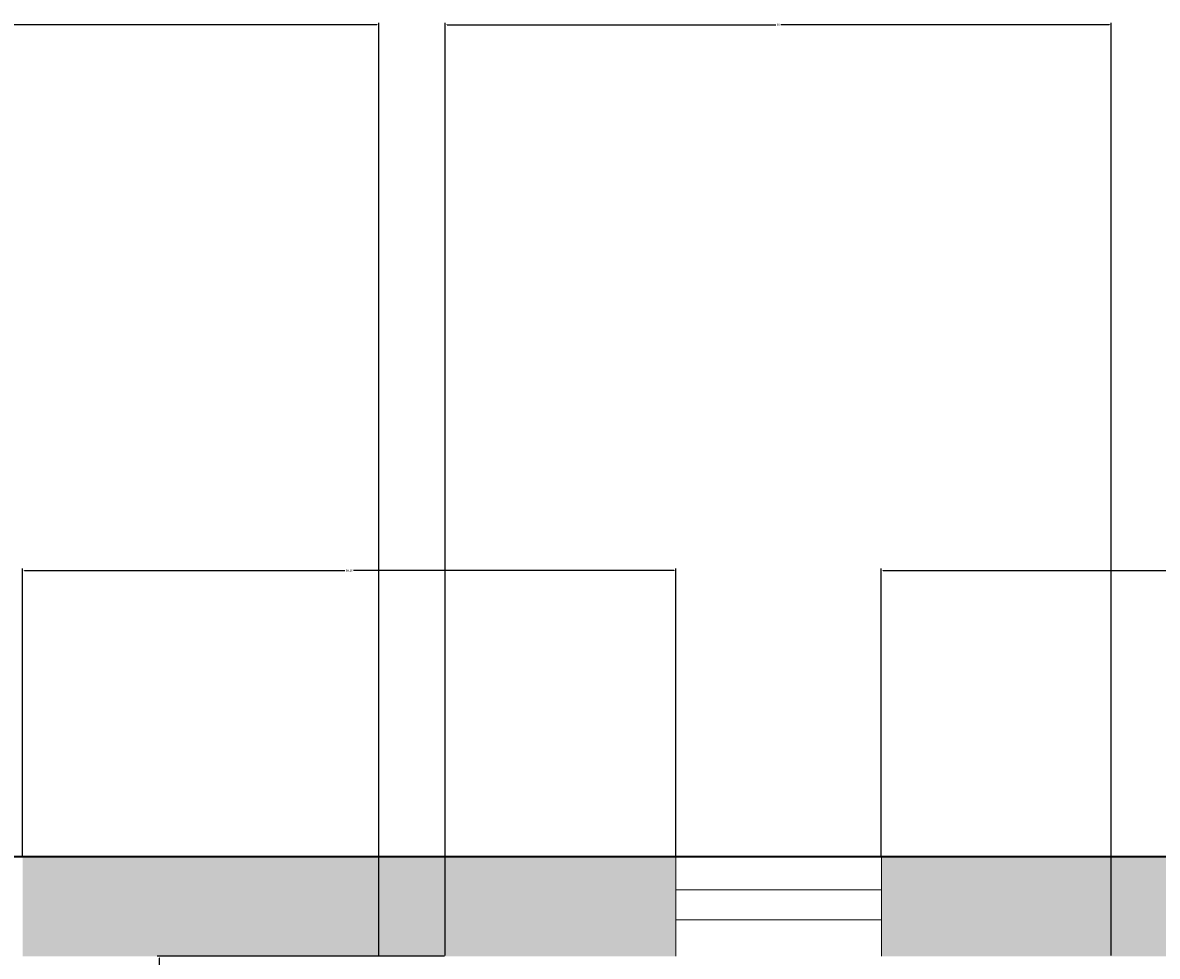
# Model space of a CAD drawing. Units: inches. Extents: x 3024 to 3952, y 1308 to 1863.
# Tile 24 of 29: x 3195 to 3297, y 1779 to 1863. Entities that reach past the tile are written whole.
import ezdxf

# ---------------------------------------------------------------- set-up
doc = ezdxf.new("R2010")
doc.units = ezdxf.units.IN
for name, color, linetype, lineweight in [('A-ANNO-DIMS', 2, 'Continuous', 18), ('A-GLAZ', 4, 'Continuous', 18), ('A-WALL', 7, 'Continuous', 35)]:
    doc.layers.add(name, color=color, linetype=linetype, lineweight=lineweight)
doc.layers.add('A-WALL-PATT', color=254, linetype='Continuous', lineweight=13, true_color=0xcecce6)
doc.styles.get("Standard").update_dxf_attribs({"font": 'arial.ttf'})
doc.dimstyles.get("Standard").update_dxf_attribs({"dimtxt": 0.18, "dimasz": 0.18, "dimexe": 0.18, "dimexo": 0.0625, "dimgap": 0.09, "dimtad": 0, "dimtih": 1, "dimtoh": 1, "dimdec": 4, "dimzin": 0, "dimdsep": 46, "dimtxsty": 'Standard', "dimcen": 0.09, "dimadec": 0, "dimazin": 0, "dimtfac": 1, "dimtdec": 4, "dimtofl": 0, "dimtmove": 0, "dimatfit": 3, "dimfxl": 1, "dimtolj": 1, "dimtzin": 0, "dimarcsym": 0})

# ---------------------------------------------------------------- blocks, each defined once
blk = doc.blocks.new('WIN-BATH-18p5IN')
for p, q in [((0, 5.99), (0, 9)), ((18.52, 6.41), (18.52, 9)), ((18.52, 6.41), (18.52, 5.99)), ((0, 3.28), (0, 0)), ((18.52, 3.69), (18.52, 0))]:
    blk.add_line(p, q)
blk.add_lwpolyline([(0, 5.99), (18.52, 5.99), (18.52, 3.28), (0, 3.28)], close=True)
blk = doc.blocks.new('*D38')
at = {"layer": 'A-ANNO-DIMS', "color": 0, "lineweight": -2, "transparency": 16777216}
for p, q in [((3106.76, 1778.67), (3106.76, 1862.78)), ((3226.76, 1778.67), (3226.76, 1862.78)), ((3106.94, 1862.6), (3166.48, 1862.6)), ((3226.58, 1862.6), (3167.04, 1862.6))]:
    blk.add_line(p, q, dxfattribs=at)
at = {"layer": 'A-ANNO-DIMS', "color": 0, "transparency": 16777216}
for points in [[(3106.94, 1862.63), (3106.94, 1862.57), (3106.76, 1862.6)], [(3226.58, 1862.63), (3226.58, 1862.57), (3226.76, 1862.6)]]:
    blk.add_solid(points, dxfattribs=at)
at = {"layer": 'Defpoints', "color": 0, "transparency": 16777216}
for p in [(3226.76, 1862.6), (3106.76, 1778.61), (3226.76, 1778.61)]:
    blk.add_point(p, dxfattribs=at)
at = {"layer": 'A-ANNO-DIMS', "color": 0, "transparency": 16777216, "insert": (3166.76, 1862.6), "char_height": 0.18, "attachment_point": 5}
blk.add_mtext('\\A1;120', dxfattribs=at)
blk = doc.blocks.new('*D39')
at = {"layer": 'A-ANNO-DIMS', "color": 0, "lineweight": -2, "transparency": 16777216}
for p, q in [((3232.76, 1778.67), (3232.76, 1862.78)), ((3292.76, 1778.67), (3292.76, 1862.78)), ((3232.94, 1862.6), (3262.54, 1862.6)), ((3292.58, 1862.6), (3262.98, 1862.6))]:
    blk.add_line(p, q, dxfattribs=at)
at = {"layer": 'A-ANNO-DIMS', "color": 0, "transparency": 16777216}
for points in [[(3232.94, 1862.63), (3232.94, 1862.57), (3232.76, 1862.6)], [(3292.58, 1862.63), (3292.58, 1862.57), (3292.76, 1862.6)]]:
    blk.add_solid(points, dxfattribs=at)
at = {"layer": 'Defpoints', "color": 0, "transparency": 16777216}
for p in [(3292.76, 1862.6), (3232.76, 1778.61), (3292.76, 1778.61)]:
    blk.add_point(p, dxfattribs=at)
at = {"layer": 'A-ANNO-DIMS', "color": 0, "transparency": 16777216, "insert": (3262.76, 1862.6), "char_height": 0.18, "attachment_point": 5}
blk.add_mtext('\\A1;60', dxfattribs=at)
blk = doc.blocks.new('*D51')
at = {"layer": 'A-ANNO-DIMS', "color": 0, "lineweight": -2, "transparency": 16777216}
for p, q in [((3232.7, 1778.61), (3206.81, 1778.61)), ((3206.99, 1778.43), (3206.99, 1736.79)), ((3206.99, 1694.79), (3206.99, 1736.42)), ((3232.7, 1694.61), (3206.81, 1694.61))]:
    blk.add_line(p, q, dxfattribs=at)
at = {"layer": 'A-ANNO-DIMS', "color": 0, "transparency": 16777216}
for points in [[(3206.96, 1778.43), (3207.02, 1778.43), (3206.99, 1778.61)], [(3206.96, 1694.79), (3207.02, 1694.79), (3206.99, 1694.61)]]:
    blk.add_solid(points, dxfattribs=at)
at = {"layer": 'Defpoints', "color": 0, "transparency": 16777216}
for p in [(3206.99, 1778.61), (3232.76, 1778.61), (3232.76, 1694.61)]:
    blk.add_point(p, dxfattribs=at)
at = {"layer": 'A-ANNO-DIMS', "color": 0, "transparency": 16777216, "insert": (3206.99, 1736.61), "char_height": 0.18, "attachment_point": 5}
blk.add_mtext('\\A1;84', dxfattribs=at)
blk = doc.blocks.new('*D72')
at = {"layer": 'A-ANNO-DIMS', "color": 0, "lineweight": -2, "transparency": 16777216}
for p, q in [((3194.68, 1787.67), (3194.68, 1813.56)), ((3194.86, 1813.38), (3223.71, 1813.38)), ((3253.35, 1813.38), (3224.5, 1813.38)), ((3253.53, 1787.67), (3253.53, 1813.56))]:
    blk.add_line(p, q, dxfattribs=at)
at = {"layer": 'A-ANNO-DIMS', "color": 0, "transparency": 16777216}
for points in [[(3194.86, 1813.41), (3194.86, 1813.35), (3194.68, 1813.38)], [(3253.35, 1813.41), (3253.35, 1813.35), (3253.53, 1813.38)]]:
    blk.add_solid(points, dxfattribs=at)
at = {"layer": 'Defpoints', "color": 0, "transparency": 16777216}
for p in [(3253.53, 1813.38), (3194.68, 1787.61), (3253.53, 1787.61)]:
    blk.add_point(p, dxfattribs=at)
at = {"layer": 'A-ANNO-DIMS', "color": 0, "transparency": 16777216, "insert": (3224.11, 1813.38), "char_height": 0.18, "attachment_point": 5}
blk.add_mtext('\\A1;58.85', dxfattribs=at)
blk = doc.blocks.new('*D73')
at = {"layer": 'A-ANNO-DIMS', "color": 0, "lineweight": -2, "transparency": 16777216}
for p, q in [((3272.05, 1787.67), (3272.05, 1813.56)), ((3272.23, 1813.38), (3302.63, 1813.38)), ((3333.68, 1813.38), (3303.28, 1813.38)), ((3333.86, 1787.67), (3333.86, 1813.56))]:
    blk.add_line(p, q, dxfattribs=at)
at = {"layer": 'A-ANNO-DIMS', "color": 0, "transparency": 16777216}
for points in [[(3272.23, 1813.41), (3272.23, 1813.35), (3272.05, 1813.38)], [(3333.68, 1813.41), (3333.68, 1813.35), (3333.86, 1813.38)]]:
    blk.add_solid(points, dxfattribs=at)
at = {"layer": 'Defpoints', "color": 0, "transparency": 16777216}
for p in [(3333.86, 1813.38), (3272.05, 1787.61), (3333.86, 1787.61)]:
    blk.add_point(p, dxfattribs=at)
at = {"layer": 'A-ANNO-DIMS', "color": 0, "transparency": 16777216, "insert": (3302.95, 1813.38), "char_height": 0.18, "attachment_point": 5}
blk.add_mtext('\\A1;61.8', dxfattribs=at)

msp = doc.modelspace()

# ---------------------------------------------------------------- hatches: boundary and pattern name
at = {"layer": 'A-WALL-PATT'}
h = msp.add_hatch(color=256, dxfattribs=at)
h.dxf.hatch_style = 1
h.paths.add_polyline_path([(3106.764, 1778.6064), (3140.5977, 1778.6064), (3140.5977, 1781.8824), (3140.5977, 1784.6), (3140.5977, 1787.6064), (3097.764, 1787.6064), (3097.764, 1590.213), (3101.04, 1590.213), (3103.7576, 1590.213), (3106.764, 1590.213)])
h.paths.add_polyline_path([(3253.5314, 1781.8824), (3253.5314, 1784.6), (3253.5314, 1787.6064), (3194.6826, 1787.6064), (3194.6826, 1785.0146), (3194.6826, 1784.6), (3194.6826, 1781.8824), (3194.6826, 1778.6064), (3253.5314, 1778.6064)])
h.paths.add_polyline_path([(3333.856, 1782.2838), (3333.856, 1784.7474), (3333.856, 1787.6064), (3272.0523, 1787.6064), (3272.0523, 1785.0146), (3272.0523, 1784.6), (3272.0523, 1781.8824), (3272.0523, 1778.6064), (3333.856, 1778.6064)])
h.paths.add_polyline_path([(3428.8344, 1784.6), (3428.8344, 1787.6064), (3378.3947, 1787.6064), (3378.3947, 1784.7474), (3378.3947, 1782.2838), (3378.3947, 1778.6064), (3428.8344, 1778.6064), (3428.8344, 1781.8824)], flags=17)
h.paths.add_polyline_path([(3469.764, 1787.6064), (3451.9386, 1787.6064), (3451.9386, 1785.0146), (3451.9386, 1784.6), (3451.9386, 1781.8824), (3451.9386, 1778.6064), (3460.764, 1778.6064), (3460.764, 1353.8452), (3277.764, 1353.8452), (3277.764, 1347.8452), (3469.764, 1347.8452), (3469.764, 1353.8452)])
h.paths.add_polyline_path([(3106.764, 1571.6922), (3104.1722, 1571.6922), (3103.7576, 1571.6922), (3101.04, 1571.6922), (3097.764, 1571.6922), (3097.764, 1347.8452), (3148.7271, 1347.8452), (3148.7271, 1351.1212), (3148.7271, 1353.8388), (3148.7271, 1356.8452), (3106.764, 1356.8452)])
h.paths.add_polyline_path([(3277.764, 1532.6064), (3262.7605, 1532.6064), (3262.7605, 1582.9359), (3256.7605, 1582.9359), (3256.7605, 1532.6064), (3244.2116, 1532.6064), (3216.238, 1532.6064), (3216.238, 1527.2064), (3216.238, 1526.6064), (3271.764, 1526.6064), (3271.764, 1356.8452), (3202.812, 1356.8452), (3202.812, 1354.2534), (3202.812, 1353.8388), (3202.812, 1351.1212), (3202.812, 1347.8452), (3277.764, 1347.8452), (3277.764, 1353.8452), (3277.764, 1356.8452)])
h.paths.add_polyline_path([(3180.238, 1532.6064), (3163.0285, 1532.6064), (3163.0285, 1531.1064), (3163.0285, 1526.6064), (3180.243, 1526.6064, -0.00416688), (3180.238, 1527.2064)])
h.paths.add_polyline_path([(3133.0285, 1531.1064, -0.01250587), (3133.066, 1532.6064), (3106.764, 1532.6064), (3106.764, 1526.6064), (3133.0285, 1526.6064)], flags=17)
h.paths.add_polyline_path([(3172.764, 1628.6064), (3166.764, 1628.6064), (3166.764, 1532.6064), (3172.764, 1532.6064)])
h.paths.add_polyline_path([(3232.764, 1649.8972), (3227.364, 1649.8972), (3226.764, 1649.8972), (3226.764, 1634.6064), (3106.764, 1634.6064), (3106.764, 1628.6064), (3232.764, 1628.6064)])

# ---------------------------------------------------------------- linework, layer by layer
at = {"layer": 'A-WALL'}
msp.add_line((3097.764, 1787.6064), (3469.764, 1787.6064), dxfattribs=at)

# ---------------------------------------------------------------- block references
at = {"layer": 'A-GLAZ'}
msp.add_blockref('WIN-BATH-18p5IN', (3253.531, 1778.606), dxfattribs=at)

# ---------------------------------------------------------------- dimensions: what is measured, and where the dimension line sits
at = {"layer": 'A-ANNO-DIMS'}
for base, p1, p2, override, picture, middle in [((3226.764, 1862.6031), (3106.764, 1778.6064), (3226.764, 1778.6064), {"dimdec": 0, "dimlfac": 1, "dimrnd": 0, "dimzin": 0, "dimdsep": 46, "dimlunit": 2}, '*D38', (3166.764, 1862.6031)), ((3292.764, 1862.6031), (3232.764, 1778.6064), (3292.764, 1778.6064), {"dimdec": 0, "dimlfac": 1, "dimrnd": 0, "dimzin": 0, "dimdsep": 46, "dimlunit": 2}, '*D39', (3262.764, 1862.6031)), ((3253.5314, 1813.3814), (3194.6826, 1787.6064), (3253.5314, 1787.6064), {"dimdec": 2, "dimlfac": 1, "dimrnd": 0, "dimzin": 0, "dimdsep": 46, "dimlunit": 2}, '*D72', (3224.107, 1813.3814)), ((3333.856, 1813.3814), (3272.0523, 1787.6064), (3333.856, 1787.6064), {"dimdec": 1, "dimlfac": 1, "dimrnd": 0, "dimzin": 0, "dimdsep": 46, "dimlunit": 2}, '*D73', (3302.9541, 1813.3814))]:
    dim = msp.add_linear_dim(base=base, p1=p1, p2=p2, dimstyle='Standard', override=override, dxfattribs=at)
    dim.commit()
    dim.dimension.update_dxf_attribs({"geometry": picture, "text_midpoint": middle})
dim = msp.add_linear_dim(base=(3206.989, 1778.6064), p1=(3232.764, 1694.6064), p2=(3232.764, 1778.6064), angle=90, dimstyle='Standard', override={"dimdec": 0, "dimlfac": 1, "dimrnd": 0, "dimzin": 0, "dimdsep": 46, "dimlunit": 2}, dxfattribs=at)
dim.commit()
dim.dimension.update_dxf_attribs({"geometry": '*D51', "text_midpoint": (3206.989, 1736.6064)})

doc.saveas('drawing.dxf')
